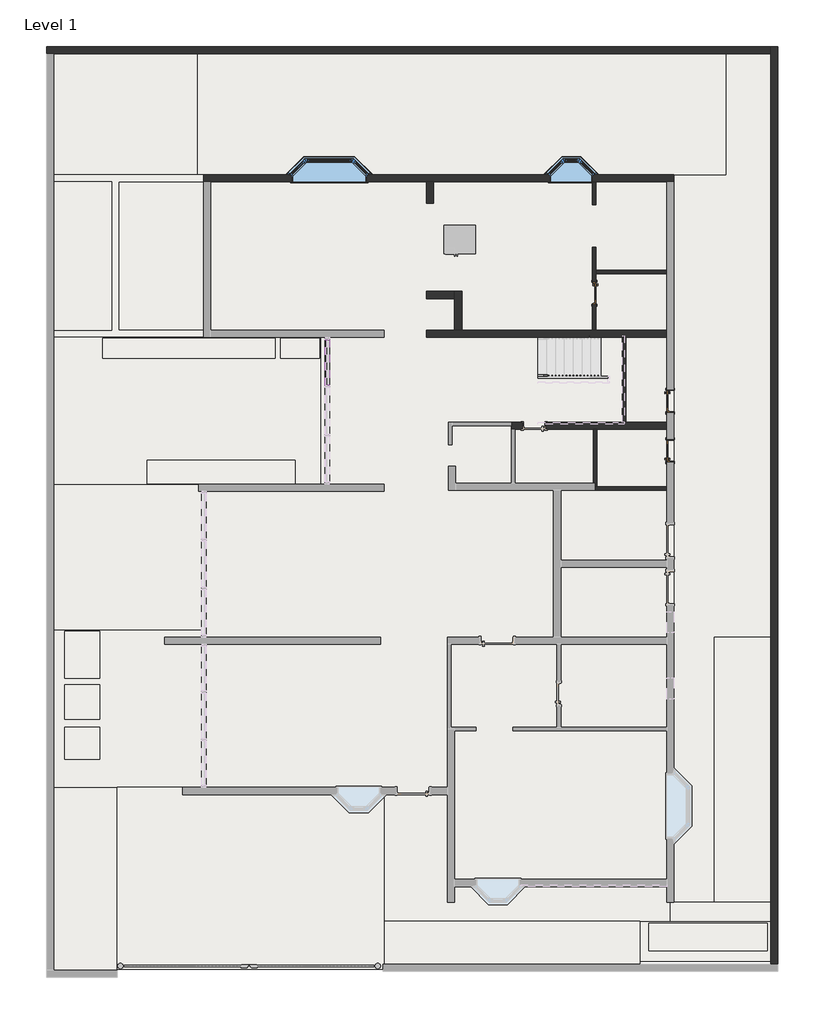
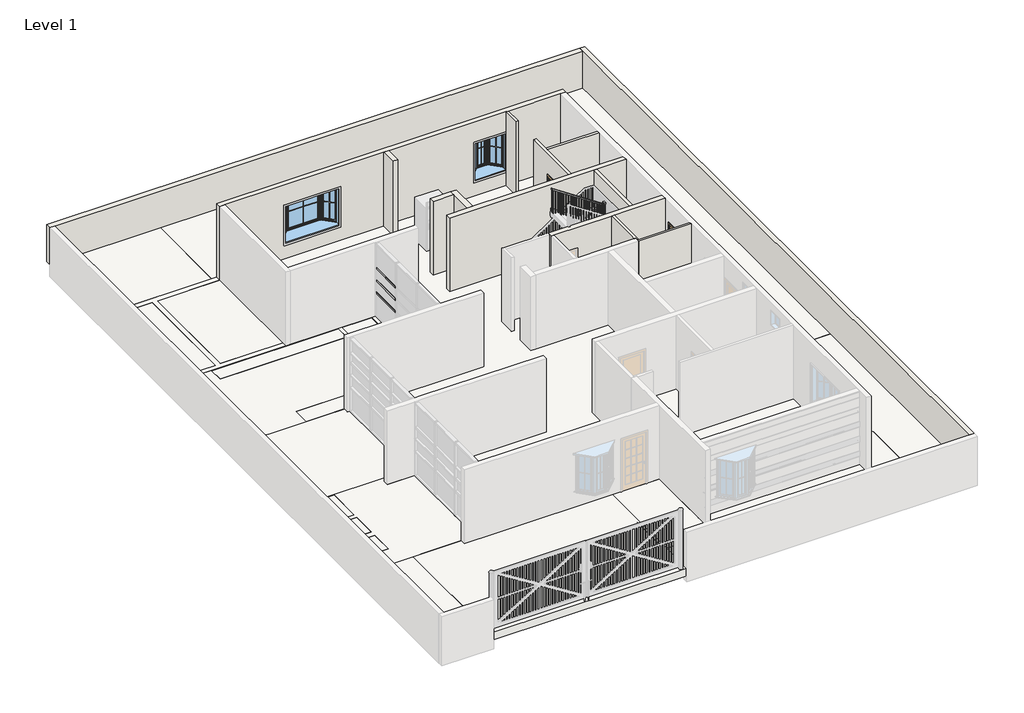
# One storey, part 4 of 5: 15 slabs, 14 walls, 3 doors, 3 members, 2 windows, 1 railing.
# Revit data of these elements (continued)
# Element 37 (IfcWindow, "Window-Bay-Casement-45_Degree_Angle : 84\" x 60\" x 18\"") (continued)
#   Materials on its faces: "Wood - Stained", "Clad - White", "Glass"
# Element 38 (IfcWindow, "Window-Bay-Casement-45_Degree_Angle : WINDOW 4'")
#   Mark = "2"
#   Interior Trim Visibility = yes
#   Exterior Trim Visibility = yes
#   Phase Created = New Construction
#   Materials on its faces: "Wood - Stained", "Clad - White", "Glass"
# Materials
#   "Cherry": class "Wood", colour RGB 226 177 128, transparency 0, Description = "Prunus Serotina", Cost = 0
#   "Aluminum": class "Metal", colour RGB 247 247 247, transparency 0, Description = "Aluminum 6061", Cost = 0
#   "GRASS TYPE": class "Generic", colour RGB 120 120 120, transparency 0, Cost = 0
#   "Concrete, Lightweight": class "Concrete", colour RGB 142 141 140, transparency 0, Description = "Lightweight concrete", Cost = 0
#   "Metal Deck": class "Metal", colour RGB 199 199 199, transparency 0, Description = "Steel, mill finish", Cost = 0
#   "MARBLE FLOOR": class "Generic", colour RGB 120 120 120, transparency 0, Cost = 0
#   "PARKING FLOORING": class "Generic", colour RGB 120 120 120, transparency 0, Cost = 0
#   "VERANDA FLOORING": class "Generic", colour RGB 120 120 120, transparency 0, Cost = 0
#   "Water": class "Liquid", colour RGB 108 195 217, transparency 0.7, Description = "Water", Cost = 0
#   "WOOD DECK 1'": class "Generic", colour RGB 120 120 120, transparency 0, Cost = 0
#   "BEIGE COLOUR": class "Generic", colour RGB 120 120 120, transparency 0, Cost = 0
#   "Wood - Stained": class "Wood", colour RGB 224 178 126, transparency 0, Cost = 0
#   "Clad - White": class "Wood", colour RGB 242 242 238, transparency 0, Cost = 0
#   "Glass": class "Glass", colour RGB 0 128 192, transparency 0.75, Description = "Soda Lime Glass", Cost = 0
